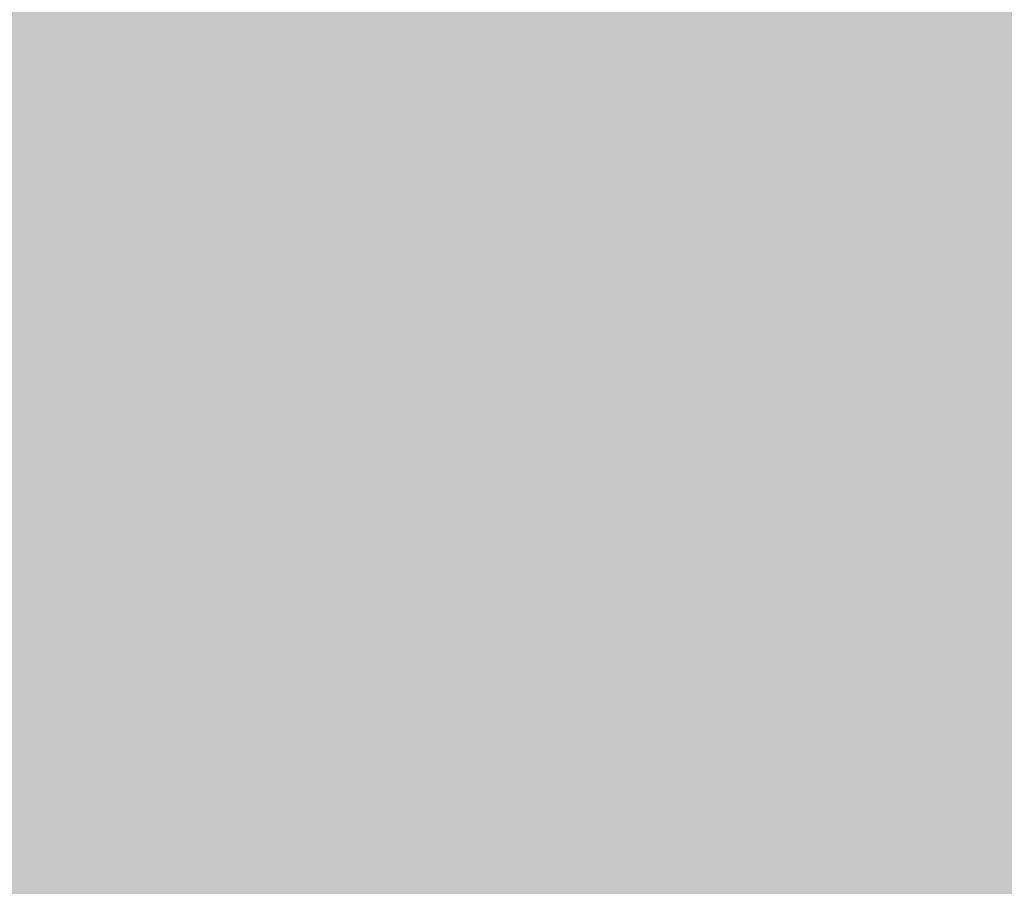
# Model space of a CAD drawing. Units: feet. Extents: x 3168 to 4724, y 827 to 1477.
# Tile 38 of 256: x 3270.273 to 3277.376, y 1087.401 to 1093.654. Entities that reach past the tile are written whole.
import ezdxf

# ---------------------------------------------------------------- set-up
doc = ezdxf.new("R2010")
doc.units = ezdxf.units.FT
doc.layers.add('A-ELEV-PATT', color=8, linetype='Continuous', lineweight=13)

msp = doc.modelspace()

# ---------------------------------------------------------------- hatches: boundary and pattern name
at = {"layer": 'A-ELEV-PATT'}
h = msp.add_hatch(color=256, dxfattribs=at)
h.dxf.hatch_style = 1
edge = h.paths.add_edge_path()
edge.add_ellipse((3552.9058, 979.2201), major_axis=(36.7449, 0), ratio=0.4848485, start_angle=0, end_angle=360)
edge = h.paths.add_edge_path()
edge.add_ellipse((3559.8916, 929.2523), major_axis=(36.7449, 0), ratio=0.4848485, start_angle=0, end_angle=360)
edge = h.paths.add_edge_path()
edge.add_line((3299.3168, 1198.6061), (3479.9167, 1198.6061))
edge.add_line((3479.9167, 1198.6061), (3479.9167, 1209.8686))
edge.add_spline(control_points=[(3479.9167, 1209.8686), (3464.3012, 1209.8686), (3448.6856, 1209.8686), (3410.9491, 1209.8686), (3388.8282, 1209.8686), (3355.6469, 1209.8686), (3344.5864, 1209.8686), (3327.9957, 1209.8686), (3322.4655, 1209.8686), (3314.1702, 1209.8686), (3311.4051, 1209.8686), (3307.2574, 1209.8686), (3305.8748, 1209.8686), (3303.801, 1209.8686), (3303.1097, 1209.8686), (3302.0728, 1209.8686), (3301.7272, 1209.8686), (3301.2087, 1209.8686), (3301.0359, 1209.8686), (3300.7767, 1209.8686), (3300.6903, 1209.8686), (3300.5606, 1209.8686), (3300.5174, 1209.8686), (3300.4526, 1209.8686), (3300.431, 1209.8686), (3300.3986, 1209.8686), (3300.3878, 1209.8686), (3300.3662, 1209.8686), (3300.3457, 1209.8686), (3300.3455, 1209.8686), (3300.3455, 1209.8686), (3300.3433, 1209.8686), (3300.3411, 1209.8686), (3300.3379, 1209.8686), (3300.3368, 1209.8686), (3300.3339, 1209.8686), (3300.3321, 1209.8686), (3300.3255, 1209.8686), (3300.3207, 1209.8686), (3300.3109, 1209.8686), (3300.306, 1209.8686), (3300.2905, 1209.8686), (3300.28, 1209.8686), (3300.2324, 1209.8688), (3300.1953, 1209.869), (3299.9511, 1209.8706), (3299.7448, 1209.8743), (3299.4368, 1209.8833), (3299.3344, 1209.8868), (3299.1811, 1209.8929), (3299.13, 1209.8951), (3298.6522, 1209.9168), (3298.2295, 1209.9457), (3297.6016, 1210.0024), (3297.3934, 1210.0235), (3297.0827, 1210.0583), (3296.9793, 1210.0705), (3296.293, 1210.1549), (3295.7181, 1210.2434), (3294.8687, 1210.3989), (3294.5877, 1210.4545), (3294.1693, 1210.5433), (3294.0304, 1210.5739), (3291.7071, 1211.1012), (3289.6536, 1211.8134), (3285.7763, 1213.564), (3283.9514, 1214.6035), (3280.5122, 1216.9801), (3278.8972, 1218.3176), (3276.3799, 1220.8295), (3275.416, 1221.9177), (3274.0393, 1223.7077), (3273.581, 1224.3495), (3273.1432, 1225.0163)], knot_values=[39.119033, 39.119033, 39.119033, 39.119033, 39.286353, 39.286353, 39.523379, 39.523379, 39.641892, 39.641892, 39.701148, 39.701148, 39.730777, 39.730777, 39.745591, 39.745591, 39.752998, 39.752998, 39.756701, 39.756701, 39.758553, 39.758553, 39.759479, 39.759479, 39.759942, 39.759942, 39.760173, 39.760173, 39.760289, 39.760289, 39.760405, 39.760405, 39.760463, 39.760463, 39.763389, 39.763389, 39.764851, 39.764851, 39.767304, 39.767304, 39.773825, 39.773825, 39.78057, 39.78057, 39.79477, 39.79477, 39.845194, 39.845194, 40.126715, 40.126715, 40.267476, 40.267476, 40.337856, 40.337856, 40.927023, 40.927023, 41.221606, 41.221606, 41.368898, 41.368898, 42.202622, 42.202622, 42.619485, 42.619485, 42.827916, 42.827916, 46.118323, 46.118323, 49.408731, 49.408731, 52.699139, 52.699139, 54.927489, 54.927489, 56.104228, 56.104228, 56.104228, 56.104228], weights=[1, 1, 1, 1, 1, 1, 1, 1, 1, 1, 1, 1, 1, 1, 1, 1, 1, 1, 1, 1, 1, 1, 1, 1, 1, 1, 1, 1, 1, 1, 1, 1, 1, 1, 1, 1, 1, 1, 1, 1, 1, 1, 1, 1, 1, 1, 1, 1, 1, 1, 1, 1, 1, 1, 1, 1, 1, 1, 1, 1, 1, 1, 1, 1, 1, 1, 1, 1, 1, 1, 1, 1, 1, 1], degree=3, periodic=0)
edge.add_line((3273.1432, 1225.0163), (3273.1432, 1099.0163))
edge.add_line((3273.1432, 1099.0163), (3299.3168, 1099.0163))
edge.add_line((3299.3168, 1099.0163), (3299.3168, 1198.6061))
edge = h.paths.add_edge_path()
edge.add_line((3304.7584, 1324.1581), (3479.9167, 1324.1581))
edge.add_line((3479.9167, 1324.1581), (3479.9167, 1335.7146))
edge.add_line((3479.9167, 1335.7146), (3269.1616, 1335.7146))
edge.add_spline(control_points=[(3269.1616, 1335.7146), (3264.0242, 1335.7146), (3258.3641, 1328.9582), (3259.2643, 1323.9003)], knot_values=[0, 0, 0, 0, 15.412191, 15.412191, 15.412191, 15.412191], degree=3, periodic=0)
edge.add_line((3259.2643, 1323.9003), (3265.5168, 1288.7691))
edge.add_line((3265.5168, 1288.7691), (3275.2651, 1261.5456))
edge.add_line((3275.2651, 1261.5456), (3304.7584, 1261.5456))
edge.add_line((3304.7584, 1261.5456), (3304.7584, 1324.1581))
h = msp.add_hatch(color=256, dxfattribs=at)
h.dxf.hatch_style = 1
h.paths.add_polyline_path([(3384.5252, 1099.0163), (3335.0292, 1099.0163), (3299.3168, 1099.0163), (3273.1432, 1099.0163), (3217.5654, 1099.0163), (3168.0693, 827.1163), (3335.0292, 827.1163)])

doc.saveas('drawing.dxf')
